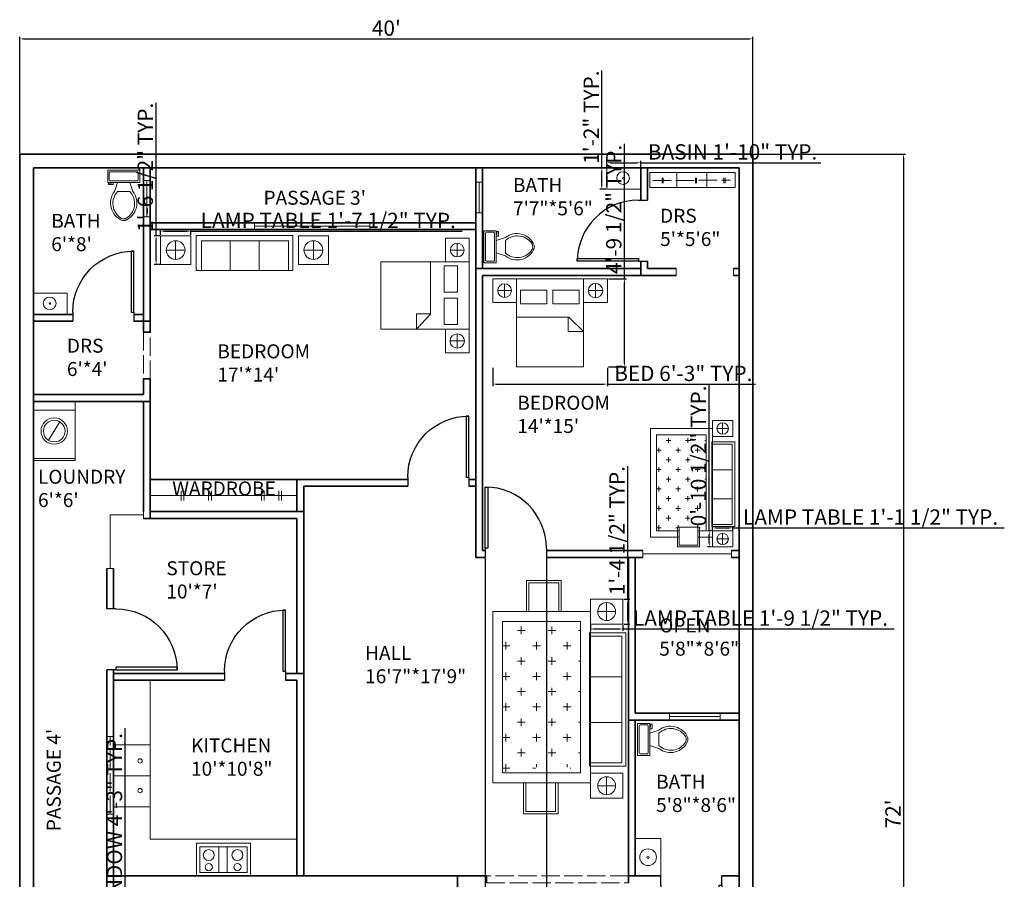
# Model space of a CAD drawing. Units: inches. Extents: x 745 to 1453, y 1850 to 2879.
# Tile 2 of 2: x 809 to 1453, y 2316 to 2879. Entities that reach past the tile are written whole.
import ezdxf

# ---------------------------------------------------------------- set-up
doc = ezdxf.new("R2010")
doc.units = ezdxf.units.IN
doc.linetypes.add('ACAD_ISO02W100', pattern=[15, 12, -3])
for name, color, linetype, lineweight in [('A-ANNO-DIMS', 210, 'Continuous', 18), ('A-AREA-IDEN', 210, 'Continuous', 18), ('A-EQPM', 140, 'Continuous', 18), ('A-FLOR-CASE', 140, 'Continuous', 20), ('A-FLOR-CASE-HIDN', 140, 'ACAD_ISO02W100', 13), ('A-FLOR-FIXT', 140, 'Continuous', 18), ('A-FURN-PATT', 140, 'Continuous', 13), ('A-GLAZ', 4, 'Continuous', 18), ('A-GLAZ-HIGH', 4, 'ACAD_ISO02W100', 18), ('A-WALL-OVHD', 92, 'ACAD_ISO02W100', 18), ('DOOR', 50, 'Continuous', 25), ('FUR', 140, 'Continuous', 18), ('WALL', 92, 'Continuous', 35)]:
    doc.layers.add(name, color=color, linetype=linetype, lineweight=lineweight)
doc.styles.get("Standard").update_dxf_attribs({"font": 'arial.ttf'})
doc.dimstyles.new('ISO-25', dxfattribs={"dimtxt": 10, "dimasz": 2.5, "dimexe": 1.25, "dimexo": 0.625, "dimtad": 1, "dimdec": 0, "dimlunit": 4, "dimtxsty": 'Standard', "dimcen": 2.5, "dimadec": 0, "dimazin": 0, "dimtfac": 1, "dimtdec": 0, "dimtmove": 0, "dimatfit": 3, "dimfxl": 1, "dimarcsym": 0})

# ---------------------------------------------------------------- blocks, each defined once
blk = doc.blocks.new('*U2')
for p, q in [((0, 0), (0, -6)), ((40, 0), (40, -6))]:
    blk.add_line(p, q)
blk.add_lwpolyline([(0, 0), (0, 40), (1.75, 40), (1.75, 0)], close=True)
blk.add_arc((0, 0), 40, 0, 90)
blk = doc.blocks.new('*U4')
for p, q in [((9.5, -6), (9.5, -2)), ((-10, -8.5), (-8, -8.5)), ((-10, -9.5), (-10, -8.5)), ((-7, -9.5), (-10, -9.5)), ((-8, -8.5), (-8, -8)), ((-7, -8), (-7, -9.5)), ((-4, -8), (-6, -14)), ((4, -8), (6, -14)), ((4, -14), (-4, -14))]:
    blk.add_line(p, q)
blk.add_lwpolyline([(10.5, -8), (10.5, 0), (-10.5, 0), (-10.5, -8)], close=True)
for points in [[(-9.5, -2), (-9.5, -6)], [(8.5, -1), (-8.5, -1)], [(-8.5, -7), (8.5, -7)]]:
    blk.add_lwpolyline(points)
for centre, radius, start, end in [((-8.62, -1.88), 0.884, 81.8699, 188.1301), ((-8.62, -6.12), 0.884, 171.8699, 278.1301), ((8.62, -1.88), 0.884, 351.8699, 98.1301), ((8.62, -6.12), 0.884, 261.8699, 8.1301), ((3.52, -21.58), 12.17, 141.46911, 247.97143), ((4.2, -21.82), 11.33, 136.36773, 238.94682), ((-3.52, -21.58), 12.17, 292.02843, 38.53071), ((-4.2, -21.82), 11.33, 301.05301, 43.63209), ((0, -27.88), 4, 245.73182, 294.26817), ((0, -29), 4, 254.86053, 285.13947)]:
    blk.add_arc(centre, radius, start, end)
blk = doc.blocks.new('*D7')
at = {"layer": 'A-ANNO-DIMS', "color": 0, "lineweight": -2, "transparency": 16777216}
for p, q in [((808.78, 2791.61), (808.78, 2867.62)), ((811.28, 2866.37), (1286.28, 2866.37)), ((1288.78, 2791.61), (1288.78, 2867.62))]:
    blk.add_line(p, q, dxfattribs=at)
at = {"layer": 'A-ANNO-DIMS', "color": 0, "lineweight": 100, "transparency": 16777216}
for points in [[(811.28, 2866.78), (811.28, 2865.95), (808.78, 2866.37)], [(1286.28, 2866.78), (1286.28, 2865.95), (1288.78, 2866.37)]]:
    blk.add_solid(points, dxfattribs=at)
at = {"layer": 'Defpoints', "color": 0, "lineweight": 100, "transparency": 16777216}
for p in [(1288.78, 2866.37), (808.78, 2790.99), (1288.78, 2790.99)]:
    blk.add_point(p, dxfattribs=at)
at = {"layer": 'A-ANNO-DIMS', "color": 0, "transparency": 16777216, "insert": (1048.78, 2872.1), "char_height": 10, "attachment_point": 5}
blk.add_mtext("40'", dxfattribs=at)
blk = doc.blocks.new('*D8')
at = {"layer": 'A-ANNO-DIMS', "color": 0, "lineweight": -2, "transparency": 16777216}
for p, q in [((1289.4, 2790.99), (1388.63, 2790.99)), ((1387.38, 2788.49), (1387.38, 1929.49)), ((1289.4, 1926.99), (1388.63, 1926.99))]:
    blk.add_line(p, q, dxfattribs=at)
at = {"layer": 'A-ANNO-DIMS', "color": 0, "lineweight": 100, "transparency": 16777216}
for points in [[(1386.96, 2788.49), (1387.79, 2788.49), (1387.38, 2790.99)], [(1386.96, 1929.49), (1387.79, 1929.49), (1387.38, 1926.99)]]:
    blk.add_solid(points, dxfattribs=at)
at = {"layer": 'Defpoints', "color": 0, "lineweight": 100, "transparency": 16777216}
for p in [(1288.78, 2790.99), (1288.78, 1926.99), (1387.38, 1926.99)]:
    blk.add_point(p, dxfattribs=at)
at = {"layer": 'A-ANNO-DIMS', "color": 0, "transparency": 16777216, "insert": (1381.73, 2358.99), "char_height": 10, "attachment_point": 5, "rotation": 90}
blk.add_mtext("72'", dxfattribs=at)
blk = doc.blocks.new('BED-DOUBLE-NIGHTSTANDS')
for p, q in [((7.78, 49.95), (7.78, 54.44)), ((7.78, 54.44), (7.78, 45.45)), ((67.29, 49.95), (67.29, 54.66)), ((67.29, 54.66), (67.29, 45.23)), ((7.78, 49.95), (3.29, 49.95)), ((3.29, 49.95), (12.28, 49.95)), ((12.28, 49.95), (7.78, 49.95)), ((67.29, 49.95), (62.57, 49.95)), ((62.57, 49.95), (72, 49.95)), ((67.29, 45.23), (67.29, 49.95)), ((15.56, 32.55), (49.81, 32.55)), ((49.81, 32.55), (59.5, 23.21)), ((49.43, 23.21), (49.43, 32.15)), ((59.5, 23.21), (49.43, 23.21))]:
    blk.add_line(p, q)
for points in [[(0, 57.67), (15.56, 57.67), (15.56, 42.22), (0, 42.22)], [(15.56, 57.67), (59.5, 57.67), (59.5, 0), (15.56, 0)], [(59.5, 57.67), (75.07, 57.67), (75.07, 42.22), (59.5, 42.22)], [(18.1, 50.16), (35.36, 50.16), (35.36, 41.34), (18.1, 41.34)], [(39.3, 50.16), (56.55, 50.16), (56.55, 41.34), (39.3, 41.34)]]:
    blk.add_lwpolyline(points, close=True)
for centre, radius in [((7.78, 49.95), 4.5), ((67.29, 49.95), 4.71)]:
    blk.add_circle(centre, radius)
blk = doc.blocks.new('LAVATORY-COMPACT')
blk.add_lwpolyline([(0, 0), (22.12, 0), (22.12, 14.01), (0, 14.01)], close=True)
for centre, radius in [((10.6, 7.23), 4.17), ((10.81, 7.15), 0.538)]:
    blk.add_circle(centre, radius)
blk = doc.blocks.new('LAMP-TABLE-BEDROOM-SM')
for p, q in [((6.75, 5.2), (6.75, 8.92)), ((6.75, 8.92), (6.75, 1.48)), ((6.75, 5.2), (3.03, 5.2)), ((3.03, 5.2), (10.47, 5.2)), ((6.75, 1.48), (6.75, 5.2))]:
    blk.add_line(p, q)
blk.add_lwpolyline([(13.5, 0), (0, 0), (0, 10.39), (13.5, 10.39)], close=True)
blk.add_circle((6.75, 5.2), 3.72)
blk = doc.blocks.new('LAMP-TABLE-BEDROOM-SQ')
for p, q in [((9.83, 9.38), (9.83, 15.51)), ((9.83, 15.51), (9.83, 3.24)), ((15.97, 9.38), (3.69, 9.38)), ((9.83, 3.24), (9.83, 9.38)), ((9.83, 9.38), (15.97, 9.38))]:
    blk.add_line(p, q)
blk.add_lwpolyline([(19.66, 18.75), (0, 18.75), (0, 0), (19.66, 0)], close=True)
blk.add_circle((9.83, 9.38), 6.14)
blk = doc.blocks.new('LAMP-TABLE-HALL')
for p, q in [((10.64, 8.19), (10.64, 14.06)), ((10.64, 14.06), (10.64, 2.33)), ((10.64, 8.19), (4.77, 8.19)), ((4.77, 8.19), (16.51, 8.19)), ((10.64, 2.33), (10.64, 8.19))]:
    blk.add_line(p, q)
blk.add_lwpolyline([(21.28, 0), (0, 0), (0, 16.39), (21.28, 16.39)], close=True)
blk.add_circle((10.64, 8.19), 5.87)
blk = doc.blocks.new('WINDOW-PASSAGE-51IN')
blk.add_line((2.25, 0), (2.25, 50.89))
blk.add_lwpolyline([(0, 50.89), (4.5, 50.89), (4.5, 0), (0, 0)], close=True)
blk = doc.blocks.new('*D20')
at = {"layer": 'A-ANNO-DIMS', "color": 0, "lineweight": -2, "transparency": 16777216}
for p, q in [((1118.44, 2650.99), (1118.44, 2639.11)), ((1193.51, 2650.99), (1193.51, 2639.11)), ((1120.94, 2640.36), (1191.01, 2640.36)), ((1193.51, 2640.36), (1290.38, 2640.36))]:
    blk.add_line(p, q, dxfattribs=at)
at = {"layer": 'A-ANNO-DIMS', "color": 0, "lineweight": 100, "transparency": 16777216}
for points in [[(1120.94, 2640.78), (1120.94, 2639.94), (1118.44, 2640.36)], [(1191.01, 2640.78), (1191.01, 2639.94), (1193.51, 2640.36)]]:
    blk.add_solid(points, dxfattribs=at)
at = {"layer": 'Defpoints', "color": 0, "lineweight": 100, "transparency": 16777216}
for p in [(1118.44, 2651.62), (1193.51, 2651.62), (1193.51, 2640.36)]:
    blk.add_point(p, dxfattribs=at)
at = {"layer": 'A-ANNO-DIMS', "color": 0, "transparency": 16777216, "insert": (1243.19, 2646.09), "char_height": 10, "attachment_point": 5}
blk.add_mtext('BED 6\'-3" TYP.', dxfattribs=at)
blk = doc.blocks.new('*D21')
at = {"layer": 'A-ANNO-DIMS', "color": 0, "lineweight": -2, "transparency": 16777216}
for p, q in [((1204.77, 2709.29), (1204.77, 2797.7)), ((1194.13, 2709.29), (1206.02, 2709.29)), ((1204.77, 2654.12), (1204.77, 2706.79)), ((1194.13, 2651.62), (1206.02, 2651.62))]:
    blk.add_line(p, q, dxfattribs=at)
at = {"layer": 'A-ANNO-DIMS', "color": 0, "lineweight": 100, "transparency": 16777216}
for points in [[(1204.35, 2706.79), (1205.19, 2706.79), (1204.77, 2709.29)], [(1204.35, 2654.12), (1205.19, 2654.12), (1204.77, 2651.62)]]:
    blk.add_solid(points, dxfattribs=at)
at = {"layer": 'Defpoints', "color": 0, "lineweight": 100, "transparency": 16777216}
for p in [(1193.51, 2709.29), (1204.77, 2709.29), (1193.51, 2651.62)]:
    blk.add_point(p, dxfattribs=at)
at = {"layer": 'A-ANNO-DIMS', "color": 0, "transparency": 16777216, "insert": (1198.97, 2754.75), "char_height": 10, "attachment_point": 5, "rotation": 90}
blk.add_mtext('4\'-9 1/2" TYP.', dxfattribs=at)
blk = doc.blocks.new('*D22')
at = {"layer": 'A-ANNO-DIMS', "color": 0, "lineweight": -2, "transparency": 16777216}
for p, q in [((1193.16, 2782.61), (1193.16, 2786.55)), ((1195.66, 2785.3), (1212.78, 2785.3)), ((1215.28, 2782.61), (1215.28, 2786.55)), ((1215.28, 2785.3), (1333.11, 2785.3))]:
    blk.add_line(p, q, dxfattribs=at)
at = {"layer": 'A-ANNO-DIMS', "color": 0, "lineweight": 100, "transparency": 16777216}
for points in [[(1195.66, 2785.72), (1195.66, 2784.89), (1193.16, 2785.3)], [(1212.78, 2785.72), (1212.78, 2784.89), (1215.28, 2785.3)]]:
    blk.add_solid(points, dxfattribs=at)
at = {"layer": 'Defpoints', "color": 0, "lineweight": 100, "transparency": 16777216}
for p in [(1215.28, 2785.3), (1193.16, 2781.99), (1215.28, 2781.99)]:
    blk.add_point(p, dxfattribs=at)
at = {"layer": 'A-ANNO-DIMS', "color": 0, "transparency": 16777216, "insert": (1275.45, 2791.1), "char_height": 10, "attachment_point": 5}
blk.add_mtext('BASIN 1\'-10" TYP.', dxfattribs=at)
blk = doc.blocks.new('*D23')
at = {"layer": 'A-ANNO-DIMS', "color": 0, "lineweight": -2, "transparency": 16777216}
for p, q in [((1189.84, 2781.99), (1189.84, 2845.75)), ((1192.53, 2781.99), (1188.59, 2781.99)), ((1189.84, 2770.48), (1189.84, 2779.49)), ((1192.53, 2767.98), (1188.59, 2767.98))]:
    blk.add_line(p, q, dxfattribs=at)
at = {"layer": 'A-ANNO-DIMS', "color": 0, "lineweight": 100, "transparency": 16777216}
for points in [[(1189.42, 2779.49), (1190.26, 2779.49), (1189.84, 2781.99)], [(1189.42, 2770.48), (1190.26, 2770.48), (1189.84, 2767.98)]]:
    blk.add_solid(points, dxfattribs=at)
at = {"layer": 'Defpoints', "color": 0, "lineweight": 100, "transparency": 16777216}
for p in [(1189.84, 2781.99), (1193.16, 2781.99), (1193.16, 2767.98)]:
    blk.add_point(p, dxfattribs=at)
at = {"layer": 'A-ANNO-DIMS', "color": 0, "transparency": 16777216, "insert": (1184.19, 2815.12), "char_height": 10, "attachment_point": 5, "rotation": 90}
blk.add_mtext('1\'-2" TYP.', dxfattribs=at)
blk = doc.blocks.new('*D24')
at = {"layer": 'A-ANNO-DIMS', "color": 0, "lineweight": -2, "transparency": 16777216}
for p, q in [((1262.2, 2544.85), (1262.2, 2547.5)), ((1264.7, 2546.25), (1273.19, 2546.25)), ((1275.69, 2544.85), (1275.69, 2547.5)), ((1275.69, 2546.25), (1453.32, 2546.25))]:
    blk.add_line(p, q, dxfattribs=at)
at = {"layer": 'A-ANNO-DIMS', "color": 0, "lineweight": 100, "transparency": 16777216}
for points in [[(1264.7, 2546.67), (1264.7, 2545.84), (1262.2, 2546.25)], [(1273.19, 2546.67), (1273.19, 2545.84), (1275.69, 2546.25)]]:
    blk.add_solid(points, dxfattribs=at)
at = {"layer": 'Defpoints', "color": 0, "lineweight": 100, "transparency": 16777216}
for p in [(1275.69, 2546.25), (1262.2, 2544.23), (1275.69, 2544.23)]:
    blk.add_point(p, dxfattribs=at)
at = {"layer": 'A-ANNO-DIMS', "color": 0, "transparency": 16777216, "insert": (1365.76, 2552.05), "char_height": 10, "attachment_point": 5}
blk.add_mtext('LAMP TABLE 1\'-1 1/2" TYP.', dxfattribs=at)
blk = doc.blocks.new('*D25')
at = {"layer": 'A-ANNO-DIMS', "color": 0, "lineweight": -2, "transparency": 16777216}
for p, q in [((1260.17, 2544.23), (1260.17, 2640)), ((1261.57, 2544.23), (1258.92, 2544.23)), ((1260.17, 2536.34), (1260.17, 2541.73)), ((1261.57, 2533.84), (1258.92, 2533.84))]:
    blk.add_line(p, q, dxfattribs=at)
at = {"layer": 'A-ANNO-DIMS', "color": 0, "lineweight": 100, "transparency": 16777216}
for points in [[(1259.76, 2541.73), (1260.59, 2541.73), (1260.17, 2544.23)], [(1259.76, 2536.34), (1260.59, 2536.34), (1260.17, 2533.84)]]:
    blk.add_solid(points, dxfattribs=at)
at = {"layer": 'Defpoints', "color": 0, "lineweight": 100, "transparency": 16777216}
for p in [(1260.17, 2544.23), (1262.2, 2544.23), (1262.2, 2533.84)]:
    blk.add_point(p, dxfattribs=at)
at = {"layer": 'A-ANNO-DIMS', "color": 0, "transparency": 16777216, "insert": (1254.38, 2593.37), "char_height": 10, "attachment_point": 5, "rotation": 90}
blk.add_mtext('0\'-10 1/2" TYP.', dxfattribs=at)
blk = doc.blocks.new('*D26')
at = {"layer": 'A-ANNO-DIMS', "color": 0, "lineweight": -2, "transparency": 16777216}
for p, q in [((901.05, 2738.12), (901.05, 2741.69)), ((903.55, 2740.44), (918.21, 2740.44)), ((920.71, 2738.12), (920.71, 2741.69)), ((920.71, 2740.44), (1098.34, 2740.44))]:
    blk.add_line(p, q, dxfattribs=at)
at = {"layer": 'A-ANNO-DIMS', "color": 0, "lineweight": 100, "transparency": 16777216}
for points in [[(903.55, 2740.86), (903.55, 2740.03), (901.05, 2740.44)], [(918.21, 2740.86), (918.21, 2740.03), (920.71, 2740.44)]]:
    blk.add_solid(points, dxfattribs=at)
at = {"layer": 'Defpoints', "color": 0, "lineweight": 100, "transparency": 16777216}
for p in [(920.71, 2740.44), (901.05, 2737.5), (920.71, 2737.5)]:
    blk.add_point(p, dxfattribs=at)
at = {"layer": 'A-ANNO-DIMS', "color": 0, "transparency": 16777216, "insert": (1010.77, 2746.24), "char_height": 10, "attachment_point": 5}
blk.add_mtext('LAMP TABLE 1\'-7 1/2" TYP.', dxfattribs=at)
blk = doc.blocks.new('*D27')
at = {"layer": 'A-ANNO-DIMS', "color": 0, "lineweight": -2, "transparency": 16777216}
for p, q in [((898.1, 2737.5), (898.1, 2824.56)), ((900.42, 2737.5), (896.85, 2737.5)), ((898.1, 2721.25), (898.1, 2735)), ((900.42, 2718.75), (896.85, 2718.75))]:
    blk.add_line(p, q, dxfattribs=at)
at = {"layer": 'A-ANNO-DIMS', "color": 0, "lineweight": 100, "transparency": 16777216}
for points in [[(897.68, 2735), (898.51, 2735), (898.1, 2737.5)], [(897.68, 2721.25), (898.51, 2721.25), (898.1, 2718.75)]]:
    blk.add_solid(points, dxfattribs=at)
at = {"layer": 'Defpoints', "color": 0, "lineweight": 100, "transparency": 16777216}
for p in [(898.1, 2737.5), (901.05, 2737.5), (901.05, 2718.75)]:
    blk.add_point(p, dxfattribs=at)
at = {"layer": 'A-ANNO-DIMS', "color": 0, "transparency": 16777216, "insert": (892.3, 2782.28), "char_height": 10, "attachment_point": 5, "rotation": 90}
blk.add_mtext('1\'-6 1/2" TYP.', dxfattribs=at)
blk = doc.blocks.new('*D28')
at = {"layer": 'A-ANNO-DIMS', "color": 0, "lineweight": -2, "transparency": 16777216}
for p, q in [((1182.37, 2482.68), (1182.37, 2478.86)), ((1203.65, 2482.68), (1203.65, 2478.86)), ((1184.87, 2480.11), (1201.15, 2480.11)), ((1203.65, 2480.11), (1381.27, 2480.11))]:
    blk.add_line(p, q, dxfattribs=at)
at = {"layer": 'A-ANNO-DIMS', "color": 0, "lineweight": 100, "transparency": 16777216}
for points in [[(1184.87, 2480.53), (1184.87, 2479.7), (1182.37, 2480.11)], [(1201.15, 2480.53), (1201.15, 2479.7), (1203.65, 2480.11)]]:
    blk.add_solid(points, dxfattribs=at)
at = {"layer": 'Defpoints', "color": 0, "lineweight": 100, "transparency": 16777216}
for p in [(1182.37, 2483.3), (1203.65, 2483.3), (1203.65, 2480.11)]:
    blk.add_point(p, dxfattribs=at)
at = {"layer": 'A-ANNO-DIMS', "color": 0, "transparency": 16777216, "insert": (1293.71, 2485.91), "char_height": 10, "attachment_point": 5}
blk.add_mtext('LAMP TABLE 1\'-9 1/2" TYP.', dxfattribs=at)
blk = doc.blocks.new('*D29')
at = {"layer": 'A-ANNO-DIMS', "color": 0, "lineweight": -2, "transparency": 16777216}
for p, q in [((1206.84, 2499.69), (1206.84, 2586.76)), ((1204.27, 2499.69), (1208.09, 2499.69)), ((1206.84, 2485.8), (1206.84, 2497.19)), ((1204.27, 2483.3), (1208.09, 2483.3))]:
    blk.add_line(p, q, dxfattribs=at)
at = {"layer": 'A-ANNO-DIMS', "color": 0, "lineweight": 100, "transparency": 16777216}
for points in [[(1206.42, 2497.19), (1207.25, 2497.19), (1206.84, 2499.69)], [(1206.42, 2485.8), (1207.25, 2485.8), (1206.84, 2483.3)]]:
    blk.add_solid(points, dxfattribs=at)
at = {"layer": 'Defpoints', "color": 0, "lineweight": 100, "transparency": 16777216}
for p in [(1203.65, 2499.69), (1206.84, 2499.69), (1203.65, 2483.3)]:
    blk.add_point(p, dxfattribs=at)
at = {"layer": 'A-ANNO-DIMS', "color": 0, "transparency": 16777216, "insert": (1201.04, 2544.47), "char_height": 10, "attachment_point": 5, "rotation": 90}
blk.add_mtext('1\'-4 1/2" TYP.', dxfattribs=at)
blk = doc.blocks.new('*D34')
at = {"layer": 'A-ANNO-DIMS', "color": 0, "lineweight": -2, "transparency": 16777216}
for p, q in [((877.91, 2284.89), (877.91, 2415.18)), ((870.9, 2284.89), (879.16, 2284.89)), ((877.91, 2236.5), (877.91, 2282.39)), ((870.9, 2234), (879.16, 2234))]:
    blk.add_line(p, q, dxfattribs=at)
at = {"layer": 'A-ANNO-DIMS', "color": 0, "lineweight": 100, "transparency": 16777216}
for points in [[(877.5, 2282.39), (878.33, 2282.39), (877.91, 2284.89)], [(877.5, 2236.5), (878.33, 2236.5), (877.91, 2234)]]:
    blk.add_solid(points, dxfattribs=at)
at = {"layer": 'Defpoints', "color": 0, "lineweight": 100, "transparency": 16777216}
for p in [(870.28, 2284.89), (877.91, 2284.89), (870.28, 2234)]:
    blk.add_point(p, dxfattribs=at)
at = {"layer": 'A-ANNO-DIMS', "color": 0, "transparency": 16777216, "insert": (872.11, 2351.28), "char_height": 10, "attachment_point": 5, "rotation": 90}
blk.add_mtext('WINDOW 4\'-3" TYP.', dxfattribs=at)
blk = doc.blocks.new('*D41')
at = {"layer": 'A-ANNO-DIMS', "color": 0, "lineweight": -2, "transparency": 16777216}
for p, q in [((1113.55, 2526.36), (1113.55, 1874.94)), ((1153.55, 2526.36), (1153.55, 1874.94)), ((1116.05, 1876.19), (1151.05, 1876.19))]:
    blk.add_line(p, q, dxfattribs=at)
at = {"layer": 'A-ANNO-DIMS', "color": 0, "lineweight": 100, "transparency": 16777216}
for points in [[(1116.05, 1876.6), (1116.05, 1875.77), (1113.55, 1876.19)], [(1151.05, 1876.6), (1151.05, 1875.77), (1153.55, 1876.19)]]:
    blk.add_solid(points, dxfattribs=at)
at = {"layer": 'Defpoints', "color": 0, "lineweight": 100, "transparency": 16777216}
for p in [(1113.55, 2526.99), (1153.55, 2526.99), (1153.55, 1876.19)]:
    blk.add_point(p, dxfattribs=at)
at = {"layer": 'A-ANNO-DIMS', "color": 0, "transparency": 16777216, "insert": (1133.55, 1881.92), "char_height": 10, "attachment_point": 5}
blk.add_mtext('3\'-4"', dxfattribs=at)

msp = doc.modelspace()

# ---------------------------------------------------------------- hatches: boundary and pattern name
at = {"layer": 'A-FURN-PATT'}
h = msp.add_hatch(dxfattribs=at)
h.set_pattern_fill('CROSS', color=256)
h.paths.add_polyline_path([(1258.13, 2607.28), (1225.73, 2607.28), (1225.73, 2544.34), (1239.36, 2544.34), (1239.36, 2546.8), (1240.38, 2546.8), (1252.77, 2546.8), (1253.83, 2546.8), (1253.83, 2544.34), (1258.13, 2544.34)])
h = msp.add_hatch(dxfattribs=at)
h.set_pattern_fill('CROSS', color=256, scale=1.576728)
h.set_pattern_definition([(0, (-807.777, -1625.891), (10.012221, 10.012221), [5.00611, -15.01833]), (90, (-805.274, -1628.394), (-10.012221, 10.012221), [5.00611, -15.01833])])
h.paths.add_polyline_path([(1124.87, 2385.84), (1146.35, 2385.84), (1146.35, 2389.72), (1147.97, 2389.72), (1167.5, 2389.72), (1169.17, 2389.72), (1169.17, 2385.84), (1175.95, 2385.84), (1175.95, 2485.09), (1124.87, 2485.09)])

# ---------------------------------------------------------------- linework, layer by layer
at = {"layer": 'A-EQPM'}
for p, q in [((817.78, 2623.41), (844.99, 2623.41)), ((835.09, 2615.65), (827.68, 2603.63)), ((831.39, 2609.64), (835.09, 2615.65)), ((817.78, 2591.78), (817.78, 2591.78)), ((817.78, 2591.78), (844.99, 2591.78))]:
    msp.add_line(p, q, dxfattribs=at)
for points in [[(817.78, 2628.99), (844.99, 2628.99), (844.99, 2590.29), (817.78, 2590.29)], [(924.42, 2339.8), (959.85, 2339.8), (959.85, 2318.49), (924.42, 2318.49)], [(926.69, 2337.53), (957.58, 2337.53), (957.58, 2320.76), (926.69, 2320.76)], [(939.23, 2337.53), (944.62, 2337.53), (944.62, 2320.76), (939.23, 2320.76)]]:
    msp.add_lwpolyline(points, close=True, dxfattribs=at)
for centre, radius in [((831.39, 2609.64), 8.64), ((831.39, 2609.64), 7.06), ((932.57, 2332.09), 3.61), ((951.33, 2332.09), 3.61), ((932.57, 2324.23), 2.34), ((951.33, 2324.23), 2.34)]:
    msp.add_circle(centre, radius, dxfattribs=at)
at = {"layer": 'A-FLOR-CASE'}
for p, q in [((1238.99, 2778.96), (1238.99, 2769.03)), ((1258.57, 2778.96), (1258.57, 2769.03)), ((914.44, 2564.24), (914.44, 2570.49)), ((914.44, 2565.76), (914.44, 2564.24)), ((916.26, 2564.24), (916.26, 2570.49)), ((932.3, 2564.24), (932.3, 2570.49)), ((934.24, 2564.24), (934.24, 2570.49)), ((967.12, 2564.24), (967.12, 2570.49)), ((968.71, 2564.24), (968.71, 2570.49)), ((978.49, 2564.24), (978.49, 2570.49)), ((980.09, 2564.24), (980.09, 2570.49)), ((870.28, 2446.49), (894.28, 2446.49)), ((894.28, 2446.49), (894.28, 2342.49)), ((990.28, 2342.49), (894.28, 2342.49)), ((990.28, 2318.49), (990.28, 2342.49))]:
    msp.add_line(p, q, dxfattribs=at)
for points in [[(1221.23, 2778.96), (1277.24, 2778.96), (1277.24, 2769.03), (1221.23, 2769.03)], [(894.28, 2556.99), (990.28, 2556.99), (990.28, 2567.49), (894.28, 2567.49)]]:
    msp.add_lwpolyline(points, close=True, dxfattribs=at)
at = {"layer": 'A-FLOR-CASE-HIDN'}
for p, q in [((1223.25, 2773.59), (1274.11, 2773.9)), ((1229.39, 2775.35), (1229.39, 2771.89)), ((1230.06, 2775.35), (1230.06, 2771.89)), ((1251.1, 2775.35), (1251.1, 2771.89)), ((1251.82, 2775.35), (1251.82, 2771.89)), ((1269.79, 2775.35), (1269.79, 2771.89)), ((1270.56, 2775.35), (1270.56, 2771.89))]:
    msp.add_line(p, q, dxfattribs=at)
at = {"layer": 'A-FLOR-FIXT'}
msp.add_line((870.28, 2383.99), (894.28, 2383.99), dxfattribs=at)
for points in [[(894.28, 2404.21), (870.28, 2404.21), (870.28, 2363.78), (894.28, 2363.78)], [(1228.51, 2318.49), (1211.78, 2318.49), (1211.78, 2342.94), (1228.51, 2342.94)]]:
    msp.add_lwpolyline(points, close=True, dxfattribs=at)
for centre, radius in [((887.59, 2393.7), 1.4), ((887.59, 2374.29), 1.4), ((1220.15, 2330.71), 5.44), ((1220.15, 2330.71), 0.775)]:
    msp.add_circle(centre, radius, dxfattribs=at)
at = {"layer": 'A-GLAZ'}
for p, q in [((892.03, 2749.89), (892.03, 2773.63)), ((1109.53, 2772.52), (1109.53, 2752.46)), ((962.52, 2743.74), (1038.02, 2743.74)), ((868.03, 2519.74), (868.03, 2554.74)), ((868.03, 2554.74), (889.78, 2554.74)), ((889.78, 2556.99), (889.78, 2552.49)), ((1216.67, 2526.99), (1216.67, 2531.49)), ((1216.67, 2529.24), (1274.72, 2529.24)), ((1274.72, 2526.99), (1274.72, 2531.49)), ((865.78, 2519.74), (870.28, 2519.74)), ((1234.13, 2422.74), (1267.25, 2422.74))]:
    msp.add_line(p, q, dxfattribs=at)
for points in [[(889.78, 2773.63), (894.28, 2773.63), (894.28, 2749.89), (889.78, 2749.89)], [(1107.28, 2772.52), (1111.78, 2772.52), (1111.78, 2752.46), (1107.28, 2752.46)], [(962.52, 2745.99), (1038.02, 2745.99), (1038.02, 2741.49), (962.52, 2741.49)], [(1234.13, 2424.99), (1267.25, 2424.99), (1267.25, 2420.49), (1234.13, 2420.49)]]:
    msp.add_lwpolyline(points, close=True, dxfattribs=at)
at = {"layer": 'A-WALL-OVHD'}
for p, q in [((1238.48, 2715.99), (1238.48, 2711.49)), ((1276.02, 2715.99), (1276.02, 2711.49))]:
    msp.add_line(p, q, dxfattribs=at)
for points in [[(889.78, 2643.93), (894.28, 2643.93), (894.28, 2674.28), (889.78, 2674.28)], [(1207.28, 2318.49), (1114.37, 2318.49), (1114.37, 2313.99), (1207.28, 2313.99)]]:
    msp.add_lwpolyline(points, close=True, dxfattribs=at)
at = {"layer": 'FUR'}
for p, q in [((924.4, 2714.79), (924.4, 2737.58)), ((924.4, 2737.58), (987.67, 2737.58)), ((946.55, 2734.15), (946.55, 2714.79)), ((965.49, 2734.15), (965.49, 2714.79)), ((987.67, 2737.58), (987.67, 2714.79)), ((927.83, 2714.79), (924.4, 2714.79)), ((987.67, 2714.79), (984.7, 2714.79)), ((1276.93, 2602.55), (1261.84, 2602.55)), ((1261.84, 2602.55), (1261.84, 2600.81)), ((1276.93, 2547.18), (1276.93, 2602.55)), ((1261.84, 2584.21), (1275.24, 2584.21)), ((1261.84, 2565.32), (1275.24, 2565.32)), ((1239.36, 2533.96), (1239.36, 2546.8)), ((1239.36, 2546.8), (1240.38, 2546.8)), ((1252.77, 2546.8), (1253.83, 2546.8)), ((1253.83, 2546.8), (1253.83, 2533.96)), ((1261.84, 2548.54), (1261.84, 2547.18)), ((1261.84, 2547.18), (1276.93, 2547.18)), ((1253.83, 2533.96), (1239.36, 2533.96)), ((1163.26, 2511.74), (1140.45, 2511.74)), ((1140.45, 2511.74), (1140.45, 2491.5)), ((1163.26, 2511.74), (1163.26, 2491.5)), ((1205.6, 2477.63), (1181.81, 2477.63)), ((1181.81, 2477.63), (1181.81, 2474.87)), ((1205.6, 2390.31), (1205.6, 2477.63)), ((1181.81, 2448.71), (1202.93, 2448.71)), ((1181.81, 2418.93), (1202.93, 2418.93)), ((1181.81, 2392.47), (1181.81, 2390.31)), ((1147.97, 2385.84), (1169.4, 2385.84)), ((1181.81, 2390.31), (1205.6, 2390.31)), ((1138.47, 2359.19), (1138.47, 2379.43)), ((1138.47, 2379.43), (1140.09, 2379.43)), ((1159.62, 2379.43), (1161.28, 2379.43)), ((1161.28, 2379.43), (1161.28, 2359.19)), ((1161.28, 2379.43), (1167.5, 2379.43)), ((1161.28, 2359.19), (1138.47, 2359.19))]:
    msp.add_line(p, q, dxfattribs=at)
for points in [[(927.83, 2734.15), (984.7, 2734.15), (984.7, 2714.79), (927.83, 2714.79)], [(1275.24, 2548.54), (1261.84, 2548.54), (1261.84, 2601.13), (1275.24, 2601.13)], [(1252.77, 2546.8), (1240.38, 2546.8), (1240.38, 2534.88), (1252.77, 2534.88)], [(1161.6, 2491.5), (1142.06, 2491.5), (1142.06, 2510.29), (1161.6, 2510.29)], [(1202.93, 2392.47), (1181.81, 2392.47), (1181.81, 2475.38), (1202.93, 2475.38)], [(1159.62, 2379.43), (1140.09, 2379.43), (1140.09, 2360.64), (1159.62, 2360.64)]]:
    msp.add_lwpolyline(points, close=True, dxfattribs=at)
for points in [[(1252.77, 2540.27), (1262.2, 2540.27), (1262.2, 2611.35), (1221.67, 2611.35), (1221.67, 2540.27), (1240.38, 2540.27)], [(1252.77, 2544.34), (1258.13, 2544.34), (1258.13, 2607.28), (1225.73, 2607.28), (1225.73, 2544.34), (1240.38, 2544.34)], [(1167.5, 2379.43), (1182.37, 2379.43), (1182.37, 2491.5), (1118.46, 2491.5), (1118.46, 2379.43), (1147.97, 2379.43)], [(1167.5, 2385.84), (1175.95, 2385.84), (1175.95, 2485.09), (1124.87, 2485.09), (1124.87, 2385.84), (1147.97, 2385.84)]]:
    msp.add_lwpolyline(points, dxfattribs=at)
at = {"layer": 'WALL'}
for p, q in [((808.78, 2790.99), (1288.78, 2790.99)), ((808.78, 1926.99), (808.78, 2790.99)), ((1288.78, 2790.99), (1288.78, 1926.99)), ((817.78, 2781.99), (1279.78, 2781.99)), ((817.78, 2781.99), (889.78, 2781.99)), ((817.78, 2193.99), (817.78, 2781.99)), ((889.78, 2781.99), (889.78, 2685.99)), ((894.28, 2781.99), (894.28, 2681.49)), ((894.28, 2781.99), (894.28, 2745.99)), ((1107.28, 2781.99), (1107.28, 2715.99)), ((1111.78, 2781.99), (1111.78, 2715.99)), ((1215.28, 2781.99), (1124.28, 2781.99)), ((1215.28, 2781.99), (1215.28, 2760.82)), ((1279.78, 2781.99), (1219.78, 2781.99)), ((1219.78, 2781.99), (1219.78, 2760.82)), ((1279.78, 2781.99), (1279.78, 1935.99)), ((894.28, 2745.99), (1107.28, 2745.99)), ((1100, 2745.99), (1107.28, 2745.99)), ((894.28, 2741.49), (1107.28, 2741.49)), ((894.28, 2741.49), (894.28, 2674.28)), ((1215.28, 2720.82), (1215.28, 2711.49)), ((1219.78, 2720.82), (1219.78, 2715.99)), ((1107.28, 2715.99), (1215.28, 2715.99)), ((1107.28, 2526.99), (1107.28, 2715.99)), ((1215.28, 2715.99), (1140, 2715.99)), ((1219.78, 2715.99), (1238.48, 2715.99)), ((1276.02, 2715.99), (1279.78, 2715.99)), ((1111.78, 2531.49), (1111.78, 2711.49)), ((1111.78, 2711.49), (1215.28, 2711.49)), ((1215.28, 2711.49), (1140, 2711.49)), ((1215.28, 2711.49), (1238.48, 2711.49)), ((1276.02, 2711.49), (1279.78, 2711.49)), ((1279.78, 2711.49), (1279.78, 2531.49)), ((889.78, 2674.28), (889.78, 2690)), ((894.28, 2674.28), (894.28, 2690)), ((843.5, 2685.99), (817.78, 2685.99)), ((817.78, 2681.49), (817.78, 2633.49)), ((843.5, 2681.49), (817.78, 2681.49)), ((889.78, 2685.99), (883.5, 2685.99)), ((894.28, 2681.49), (883.5, 2681.49)), ((889.78, 2633.49), (889.78, 2643.93)), ((894.28, 2628.99), (894.28, 2643.93)), ((894.28, 2643.93), (894.28, 2573.49)), ((817.78, 2633.49), (889.78, 2633.49)), ((817.78, 2628.99), (894.28, 2628.99)), ((817.78, 2628.99), (817.78, 2556.99)), ((889.78, 2556.99), (889.78, 2628.99)), ((894.28, 2552.49), (894.28, 2628.99)), ((990.28, 2577.99), (894.28, 2577.99)), ((990.28, 2577.99), (1062.81, 2577.99)), ((990.28, 2556.99), (990.28, 2577.99)), ((994.78, 2573.49), (1062.81, 2573.49)), ((994.78, 2556.99), (994.78, 2573.49)), ((1102.81, 2577.99), (1107.28, 2577.99)), ((1102.81, 2573.49), (1107.28, 2573.49)), ((889.78, 2552.49), (894.28, 2552.49)), ((894.28, 2556.99), (994.78, 2556.99)), ((894.28, 2552.49), (990.28, 2552.49)), ((990.28, 2552.49), (990.28, 2520.13)), ((994.78, 2556.99), (994.78, 2520.13)), ((990.28, 2450.99), (990.28, 2534.99)), ((994.78, 2450.99), (994.78, 2534.99)), ((1113.55, 2526.99), (1107.28, 2526.99)), ((1113.55, 2531.49), (1111.78, 2531.49)), ((1216.67, 2531.49), (1153.55, 2531.49)), ((1216.67, 2526.99), (1153.55, 2526.99)), ((1207.28, 2420.49), (1207.28, 2526.99)), ((1211.78, 2424.99), (1211.78, 2526.99)), ((1279.78, 2531.49), (1274.72, 2531.49)), ((1279.78, 2526.99), (1274.72, 2526.99)), ((1279.78, 2526.99), (1279.78, 2424.99)), ((865.78, 2519.74), (865.78, 2493.25)), ((870.28, 2519.74), (870.28, 2493.25)), ((865.78, 2453.25), (865.78, 2189.49)), ((870.28, 2453.25), (870.28, 2189.49)), ((870.28, 2450.99), (942.81, 2450.99)), ((942.81, 2450.99), (870.28, 2450.99)), ((994.78, 2450.99), (982.81, 2450.99)), ((982.81, 2450.99), (990.28, 2450.99)), ((994.78, 2318.49), (994.78, 2450.99)), ((942.81, 2446.49), (870.28, 2446.49)), ((990.28, 2446.49), (982.81, 2446.49)), ((990.28, 2318.49), (990.28, 2446.49)), ((1279.78, 2424.99), (1211.78, 2424.99)), ((1279.78, 2420.49), (1207.28, 2420.49)), ((1207.28, 2313.99), (1207.28, 2420.49)), ((1211.78, 2318.49), (1211.78, 2420.49)), ((1279.78, 2420.49), (1279.78, 2318.49)), ((870.28, 2318.49), (1086.28, 2318.49)), ((870.28, 2318.49), (990.28, 2318.49)), ((1086.28, 2318.49), (1095.28, 2318.49)), ((1095.28, 2318.49), (1095.28, 2189.49)), ((1114.37, 2318.49), (1095.28, 2318.49)), ((1114.37, 2313.99), (1114.37, 2318.49)), ((1228.51, 2318.49), (1207.28, 2318.49)), ((1228.51, 2318.49), (1211.78, 2318.49)), ((1279.78, 2318.49), (1268.51, 2318.49)), ((1279.78, 2318.49), (1268.51, 2318.49))]:
    msp.add_line(p, q, dxfattribs=at)
for points in [[(889.78, 2674.28), (894.28, 2674.28)], [(894.28, 2643.93), (889.78, 2643.93)]]:
    msp.add_lwpolyline(points, dxfattribs=at)

# ---------------------------------------------------------------- block references
at = {"layer": 'A-FLOR-FIXT'}
for name, p in [('*U4', (876.89, 2780.43)), ('LAVATORY-COMPACT', (1193.16, 2767.98)), ('LAVATORY-COMPACT', (817.78, 2685.99))]:
    msp.add_blockref(name, p, dxfattribs=at)
at = {"layer": 'A-FLOR-FIXT', "xscale": -1, "rotation": 90}
for p in [(1112.7, 2730.28), (1213.25, 2407.83)]:
    msp.add_blockref('*U4', p, dxfattribs=at)
at = {"layer": 'A-GLAZ-HIGH'}
msp.add_blockref('WINDOW-PASSAGE-51IN', (865.78, 2358.77), dxfattribs=at)
at = {"layer": 'DOOR'}
for p, rotation in [((1213.78, 2720.82), 90), ((1268.51, 2312.49), 180)]:
    msp.add_blockref('*U2', p, dxfattribs=dict(at, rotation=rotation))
at = {"layer": 'DOOR', "xscale": -1}
for p in [(883.5, 2687.49), (1102.81, 2579.49), (982.81, 2452.49)]:
    msp.add_blockref('*U2', p, dxfattribs=at)
at = {"layer": 'DOOR'}
msp.add_blockref('*U2', (1113.55, 2532.99), dxfattribs=at)
at = {"layer": 'DOOR', "xscale": -1, "rotation": 270}
msp.add_blockref('*U2', (871.78, 2453.25), dxfattribs=at)
at = {"layer": 'FUR'}
for name, p in [('LAMP-TABLE-BEDROOM-SQ', (901.05, 2718.74)), ('LAMP-TABLE-BEDROOM-SQ', (991.19, 2718.74)), ('BED-DOUBLE-NIGHTSTANDS', (1118.44, 2651.62)), ('LAMP-TABLE-BEDROOM-SM', (1262.2, 2606.15)), ('LAMP-TABLE-BEDROOM-SM', (1262.2, 2533.84)), ('LAMP-TABLE-HALL', (1182.37, 2483.31)), ('LAMP-TABLE-HALL', (1182.37, 2369.28))]:
    msp.add_blockref(name, p, dxfattribs=at)
at = {"layer": 'FUR', "rotation": 269.9999999999993}
msp.add_blockref('BED-DOUBLE-NIGHTSTANDS', (1045.25, 2735.89), dxfattribs=at)

# ---------------------------------------------------------------- texts
at = {"layer": 'A-AREA-IDEN', "attachment_point": 1}
for s, insert, char_height in [('BATH\\P7\'7"*5\'6"', (1131.68, 2775.24), 9.145), ("PASSAGE 3'", (968.38, 2766.92), 9.145), ('DRS\\P5\'*5\'6"', (1228.01, 2755.15), 9.145), ("BATH\\P6'*8'", (829.42, 2751.82), 9.145), ("DRS\\P6'*4'", (839.68, 2670.08), 9.145), ("BEDROOM\\P17'*14'", (938.18, 2666.41), 9.145), ("BEDROOM\\P14'*15'", (1134.53, 2632.76), 9.145), ("LOUNDRY\\P6'*6'", (820.78, 2584.3), 9.145), ('WARDROBE', (908.64, 2576.65), 9.145), ("STORE\\P10'*7'", (904.8, 2524.43), 9.145), ('OPEN\\P5\'8"*8\'6"', (1227.43, 2487.01), 9.145), ('HALL\\P16\'7"*17\'9"', (1034.91, 2468.96), 9.1453), ('KITCHEN\\P10\'*10\'8"', (920.95, 2408.41), 9.145), ('BATH\\P5\'8"*8\'6"', (1225.38, 2384.68), 9.145)]:
    msp.add_mtext_dynamic_manual_height_columns(s, width=282.6971, gutter_width=45.73, heights=[0], dxfattribs=dict(at, insert=insert, char_height=char_height))
at = {"layer": 'A-AREA-IDEN', "insert": (826.49, 2347.71), "char_height": 9.145, "attachment_point": 1, "rotation": 90}
msp.add_mtext_dynamic_manual_height_columns("PASSAGE 4'", width=282.6971, gutter_width=45.73, heights=[0], dxfattribs=at)

# ---------------------------------------------------------------- dimensions: what is measured, and where the dimension line sits
at = {"layer": 'A-ANNO-DIMS'}
for base, p1, p2, override, picture, middle in [((1288.78, 2866.37), (808.78, 2790.99), (1288.78, 2790.99), {"dimclrd": 0, "dimclre": 0, "dimclrt": 0}, '*D7', (1048.78, 2872.1)), ((1153.55, 1876.19), (1113.55, 2526.99), (1153.55, 2526.99), {"dimdec": 1, "dimlfac": 1, "dimrnd": 0, "dimzin": 1, "dimdsep": 46, "dimlunit": 4, "dimfrac": 2}, '*D41', (1133.55, 1881.92))]:
    dim = msp.add_linear_dim(base=base, p1=p1, p2=p2, dimstyle='ISO-25', override=override, dxfattribs=at)
    dim.commit()
    dim.dimension.update_dxf_attribs({"geometry": picture, "text_midpoint": middle})
for base, p1, p2, text, picture, middle in [((1189.84, 2781.99), (1193.16, 2767.98), (1193.16, 2781.99), '<> TYP.', '*D23', (1184.19, 2815.12)), ((898.09777, 2737.49525), (901.04744, 2718.74531), (901.04744, 2737.49525), '<> TYP.', '*D27', (892.30224, 2782.27782)), ((1204.77, 2709.29), (1193.51, 2651.62), (1193.51, 2709.29), '<> TYP.', '*D21', (1198.97, 2754.75)), ((1260.17, 2544.23), (1262.2, 2533.84), (1262.2, 2544.23), '<> TYP.', '*D25', (1254.38, 2593.37)), ((1206.84, 2499.69), (1203.65, 2483.3), (1203.65, 2499.69), '<> TYP.', '*D29', (1201.04, 2544.47)), ((877.91, 2284.89), (870.28, 2234), (870.28, 2284.89), 'WINDOW <> TYP.', '*D34', (872.11, 2351.28))]:
    dim = msp.add_linear_dim(base=base, p1=p1, p2=p2, angle=90, text=text, dimstyle='ISO-25', override={"dimdec": 1, "dimlfac": 1, "dimrnd": 0, "dimzin": 1, "dimdsep": 46, "dimlunit": 4, "dimfrac": 2}, dxfattribs=at)
    dim.commit()
    dim.dimension.update_dxf_attribs({"geometry": picture, "text_midpoint": middle})
for base, p1, p2, text, picture, middle in [((1215.28, 2785.3), (1193.16, 2781.99), (1215.28, 2781.99), 'BASIN <> TYP.', '*D22', (1275.45, 2791.1)), ((920.71, 2740.44), (901.05, 2737.5), (920.71, 2737.5), 'LAMP TABLE <> TYP.', '*D26', (1010.77, 2746.24)), ((1193.51, 2640.36), (1118.44, 2651.62), (1193.51, 2651.62), 'BED <> TYP.', '*D20', (1243.19, 2646.09)), ((1275.69, 2546.25), (1262.2, 2544.23), (1275.69, 2544.23), 'LAMP TABLE <> TYP.', '*D24', (1365.76, 2552.05)), ((1203.65, 2480.11), (1182.37, 2483.3), (1203.65, 2483.3), 'LAMP TABLE <> TYP.', '*D28', (1293.71, 2485.91))]:
    dim = msp.add_linear_dim(base=base, p1=p1, p2=p2, text=text, dimstyle='ISO-25', override={"dimdec": 1, "dimlfac": 1, "dimrnd": 0, "dimzin": 1, "dimdsep": 46, "dimlunit": 4, "dimfrac": 2}, dxfattribs=at)
    dim.commit()
    dim.dimension.update_dxf_attribs({"geometry": picture, "text_midpoint": middle})
dim = msp.add_linear_dim(base=(1387.38, 1926.99), p1=(1288.78, 2790.99), p2=(1288.78, 1926.99), angle=90, dimstyle='ISO-25', override={"dimclrd": 0, "dimclre": 0, "dimclrt": 0}, dxfattribs=at)
dim.commit()
dim.dimension.update_dxf_attribs({"geometry": '*D8', "text_midpoint": (1381.73, 2358.99)})

doc.saveas('drawing.dxf')
